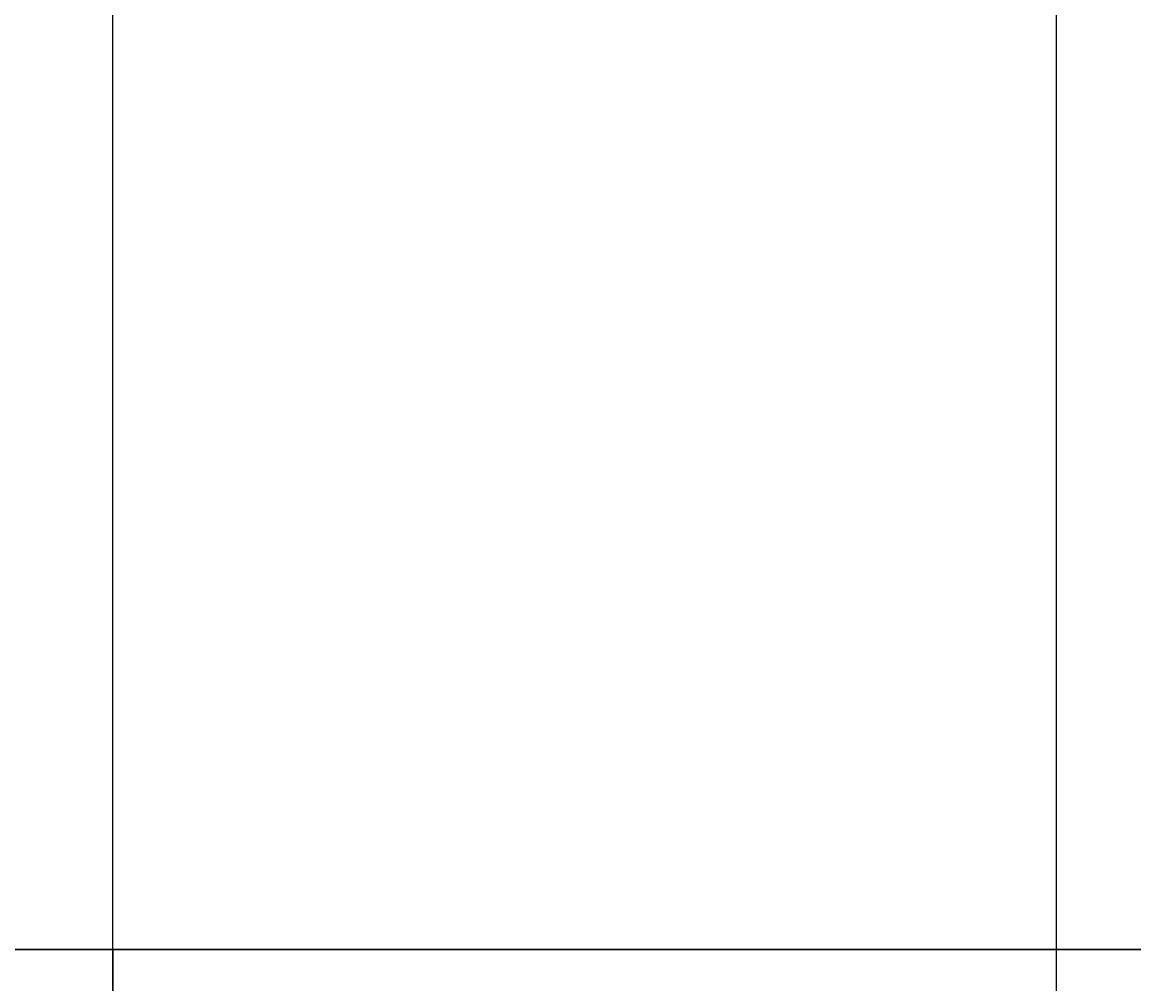
# Model space of a CAD drawing. Units: feet. Extents: x 105 to 1094, y -88 to 588.
# Tile 47 of 59: x 551 to 575, y 470 to 492. Entities that reach past the tile are written whole.
import ezdxf

# ---------------------------------------------------------------- set-up
doc = ezdxf.new("R2010")
doc.units = ezdxf.units.FT
doc.header["$MEASUREMENT"] = 0
doc.layers.add('A-ANNO-DIMS', color=2, linetype='Continuous', lineweight=18)
doc.layers.add('A-FLOR-PROJ', color=8, linetype='Continuous', lineweight=25)
doc.styles.get("Standard").update_dxf_attribs({"font": 'arial.ttf'})
doc.dimstyles.get("Standard").update_dxf_attribs({"dimtxt": 0.18, "dimasz": 0.18, "dimexe": 0.18, "dimexo": 0.0625, "dimgap": 0.09, "dimtad": 0, "dimtih": 1, "dimtoh": 1, "dimdec": 4, "dimzin": 0, "dimdsep": 46, "dimtxsty": 'Standard', "dimcen": 0.09, "dimadec": 0, "dimazin": 0, "dimtfac": 1, "dimtdec": 4, "dimtofl": 0, "dimtmove": 0, "dimatfit": 3, "dimfxl": 1, "dimtolj": 1, "dimtzin": 0, "dimarcsym": 0})

# ---------------------------------------------------------------- blocks, each defined once
blk = doc.blocks.new('*D21')
at = {"layer": 'A-ANNO-DIMS', "color": 0, "lineweight": -2, "transparency": 16777216}
for p, q in [((849.626, 543.081), (105.458, 543.081)), ((105.638, 542.901), (105.638, 250.263)), ((105.638, -42.739), (105.638, 249.899)), ((849.626, -42.919), (105.458, -42.919))]:
    blk.add_line(p, q, dxfattribs=at)
at = {"layer": 'A-ANNO-DIMS', "color": 0, "transparency": 16777216}
for points in [[(105.608, 542.901), (105.668, 542.901), (105.638, 543.081)], [(105.608, -42.739), (105.668, -42.739), (105.638, -42.919)]]:
    blk.add_solid(points, dxfattribs=at)
at = {"layer": 'Defpoints', "color": 0, "transparency": 16777216}
for p in [(105.638, 543.081), (849.688, 543.081), (849.688, -42.919)]:
    blk.add_point(p, dxfattribs=at)
at = {"layer": 'A-ANNO-DIMS', "color": 0, "transparency": 16777216, "insert": (105.638, 250.081), "char_height": 0.18, "attachment_point": 5}
blk.add_mtext('\\A1;586', dxfattribs=at)
blk = doc.blocks.new('*D25')
at = {"layer": 'A-ANNO-DIMS', "color": 0, "lineweight": -2, "transparency": 16777216}
for p, q in [((438.688, 527.144), (438.688, 588.311)), ((552.688, 471.144), (552.688, 588.311)), ((438.868, 588.131), (495.408, 588.131)), ((552.508, 588.131), (495.968, 588.131))]:
    blk.add_line(p, q, dxfattribs=at)
at = {"layer": 'A-ANNO-DIMS', "color": 0, "transparency": 16777216}
for points in [[(438.868, 588.161), (438.868, 588.101), (438.688, 588.131)], [(552.508, 588.161), (552.508, 588.101), (552.688, 588.131)]]:
    blk.add_solid(points, dxfattribs=at)
at = {"layer": 'Defpoints', "color": 0, "transparency": 16777216}
for p in [(552.688, 588.131), (438.688, 527.081), (552.688, 471.081)]:
    blk.add_point(p, dxfattribs=at)
at = {"layer": 'A-ANNO-DIMS', "color": 0, "transparency": 16777216, "insert": (495.688, 588.131), "char_height": 0.18, "attachment_point": 5}
blk.add_mtext('\\A1;114', dxfattribs=at)
blk = doc.blocks.new('*D26')
at = {"layer": 'A-ANNO-DIMS', "color": 0, "lineweight": -2, "transparency": 16777216}
for p, q in [((552.688, 471.144), (552.688, 588.311)), ((646.688, 471.144), (646.688, 588.311)), ((552.868, 588.131), (599.47, 588.131)), ((646.508, 588.131), (599.907, 588.131))]:
    blk.add_line(p, q, dxfattribs=at)
at = {"layer": 'A-ANNO-DIMS', "color": 0, "transparency": 16777216}
for points in [[(552.868, 588.161), (552.868, 588.101), (552.688, 588.131)], [(646.508, 588.161), (646.508, 588.101), (646.688, 588.131)]]:
    blk.add_solid(points, dxfattribs=at)
at = {"layer": 'Defpoints', "color": 0, "transparency": 16777216}
for p in [(646.688, 588.131), (552.688, 471.081), (646.688, 471.081)]:
    blk.add_point(p, dxfattribs=at)
at = {"layer": 'A-ANNO-DIMS', "color": 0, "transparency": 16777216, "insert": (599.688, 588.131), "char_height": 0.18, "attachment_point": 5}
blk.add_mtext('\\A1;94', dxfattribs=at)
blk = doc.blocks.new('*D31')
at = {"layer": 'A-ANNO-DIMS', "color": 0, "lineweight": -2, "transparency": 16777216}
for p, q in [((438.751, 527.081), (1093.918, 527.081)), ((1093.738, 526.901), (1093.738, 499.263)), ((1093.738, 471.261), (1093.738, 498.899)), ((438.751, 471.081), (1093.918, 471.081))]:
    blk.add_line(p, q, dxfattribs=at)
at = {"layer": 'A-ANNO-DIMS', "color": 0, "transparency": 16777216}
for points in [[(1093.708, 526.901), (1093.768, 526.901), (1093.738, 527.081)], [(1093.708, 471.261), (1093.768, 471.261), (1093.738, 471.081)]]:
    blk.add_solid(points, dxfattribs=at)
at = {"layer": 'Defpoints', "color": 0, "transparency": 16777216}
for p in [(438.688, 527.081), (1093.738, 527.081), (438.688, 471.081)]:
    blk.add_point(p, dxfattribs=at)
at = {"layer": 'A-ANNO-DIMS', "color": 0, "transparency": 16777216, "insert": (1093.738, 499.081), "char_height": 0.18, "attachment_point": 5}
blk.add_mtext('\\A1;56', dxfattribs=at)
blk = doc.blocks.new('*D32')
at = {"layer": 'A-ANNO-DIMS', "color": 0, "lineweight": -2, "transparency": 16777216}
for p, q in [((646.626, 471.081), (105.458, 471.081)), ((105.638, 470.901), (105.638, 456.263)), ((105.638, 441.261), (105.638, 455.899)), ((646.626, 441.081), (105.458, 441.081))]:
    blk.add_line(p, q, dxfattribs=at)
at = {"layer": 'A-ANNO-DIMS', "color": 0, "transparency": 16777216}
for points in [[(105.608, 470.901), (105.668, 470.901), (105.638, 471.081)], [(105.608, 441.261), (105.668, 441.261), (105.638, 441.081)]]:
    blk.add_solid(points, dxfattribs=at)
at = {"layer": 'Defpoints', "color": 0, "transparency": 16777216}
for p in [(105.638, 471.081), (646.688, 471.081), (646.688, 441.081)]:
    blk.add_point(p, dxfattribs=at)
at = {"layer": 'A-ANNO-DIMS', "color": 0, "transparency": 16777216, "insert": (105.638, 456.081), "char_height": 0.18, "attachment_point": 5}
blk.add_mtext('\\A1;30', dxfattribs=at)
blk = doc.blocks.new('*D47')
at = {"layer": 'A-ANNO-DIMS', "color": 0, "lineweight": -2, "transparency": 16777216}
for p, q in [((552.688, 441.144), (552.688, 588.311)), ((573.483, 441.144), (573.483, 588.311)), ((552.868, 588.131), (562.621, 588.131)), ((573.303, 588.131), (563.55, 588.131))]:
    blk.add_line(p, q, dxfattribs=at)
at = {"layer": 'A-ANNO-DIMS', "color": 0, "transparency": 16777216}
for points in [[(552.868, 588.161), (552.868, 588.101), (552.688, 588.131)], [(573.303, 588.161), (573.303, 588.101), (573.483, 588.131)]]:
    blk.add_solid(points, dxfattribs=at)
at = {"layer": 'Defpoints', "color": 0, "transparency": 16777216}
for p in [(573.483, 588.131), (552.688, 441.081), (573.483, 441.081)]:
    blk.add_point(p, dxfattribs=at)
at = {"layer": 'A-ANNO-DIMS', "color": 0, "transparency": 16777216, "insert": (563.085, 588.131), "char_height": 0.18, "attachment_point": 5}
blk.add_mtext('\\A1;20.794', dxfattribs=at)
blk = doc.blocks.new('*D48')
at = {"layer": 'A-ANNO-DIMS', "color": 0, "lineweight": -2, "transparency": 16777216}
for p, q in [((573.483, 441.144), (573.483, 588.311)), ((633.483, 441.144), (633.483, 588.311)), ((573.663, 588.131), (603.263, 588.131)), ((633.303, 588.131), (603.702, 588.131))]:
    blk.add_line(p, q, dxfattribs=at)
at = {"layer": 'A-ANNO-DIMS', "color": 0, "transparency": 16777216}
for points in [[(573.663, 588.161), (573.663, 588.101), (573.483, 588.131)], [(633.303, 588.161), (633.303, 588.101), (633.483, 588.131)]]:
    blk.add_solid(points, dxfattribs=at)
at = {"layer": 'Defpoints', "color": 0, "transparency": 16777216}
for p in [(633.483, 588.131), (573.483, 441.081), (633.483, 441.081)]:
    blk.add_point(p, dxfattribs=at)
at = {"layer": 'A-ANNO-DIMS', "color": 0, "transparency": 16777216, "insert": (603.483, 588.131), "char_height": 0.18, "attachment_point": 5}
blk.add_mtext('\\A1;60', dxfattribs=at)

msp = doc.modelspace()

# ---------------------------------------------------------------- linework, layer by layer
at = {"layer": 'A-FLOR-PROJ'}
for p, q in [((438.6883, 471.0812), (552.6883, 471.0812)), ((552.6883, 471.0812), (552.6883, 441.0812))]:
    msp.add_line(p, q, dxfattribs=at)

# ---------------------------------------------------------------- dimensions: what is measured, and where the dimension line sits
at = {"layer": 'A-ANNO-DIMS'}
for base, p1, p2, override, picture, middle in [((552.6883, 588.1312), (438.6883, 527.0812), (552.6883, 471.0812), {"dimdec": 0, "dimlfac": 1, "dimrnd": 0, "dimzin": 0, "dimdsep": 46, "dimlunit": 2}, '*D25', (495.6883, 588.1312)), ((646.6883, 588.1312), (552.6883, 471.0812), (646.6883, 471.0812), {"dimdec": 0, "dimlfac": 1, "dimrnd": 0, "dimzin": 0, "dimdsep": 46, "dimlunit": 2}, '*D26', (599.6883, 588.1312)), ((573.4826, 588.1312), (552.6883, 441.0812), (573.4826, 441.0812), {"dimdec": 3, "dimlfac": 1, "dimrnd": 0, "dimzin": 0, "dimdsep": 46, "dimlunit": 2}, '*D47', (563.0854, 588.1312)), ((633.4826, 588.1312), (573.4826, 441.0812), (633.4826, 441.0812), {"dimdec": 0, "dimlfac": 1, "dimrnd": 0, "dimzin": 0, "dimdsep": 46, "dimlunit": 2}, '*D48', (603.4826, 588.1312))]:
    dim = msp.add_linear_dim(base=base, p1=p1, p2=p2, dimstyle='Standard', override=override, dxfattribs=at)
    dim.commit()
    dim.dimension.update_dxf_attribs({"geometry": picture, "text_midpoint": middle})
for base, p1, p2, picture, middle in [((105.6383, 543.0812), (849.6883, -42.9188), (849.6883, 543.0812), '*D21', (105.6383, 250.0812)), ((1093.7383, 527.0812), (438.6883, 471.0812), (438.6883, 527.0812), '*D31', (1093.7383, 499.0812)), ((105.6383, 471.0812), (646.6883, 441.0812), (646.6883, 471.0812), '*D32', (105.6383, 456.0812))]:
    dim = msp.add_linear_dim(base=base, p1=p1, p2=p2, angle=90, dimstyle='Standard', override={"dimdec": 0, "dimlfac": 1, "dimrnd": 0, "dimzin": 0, "dimdsep": 46, "dimlunit": 2}, dxfattribs=at)
    dim.commit()
    dim.dimension.update_dxf_attribs({"geometry": picture, "text_midpoint": middle})

doc.saveas('drawing.dxf')
